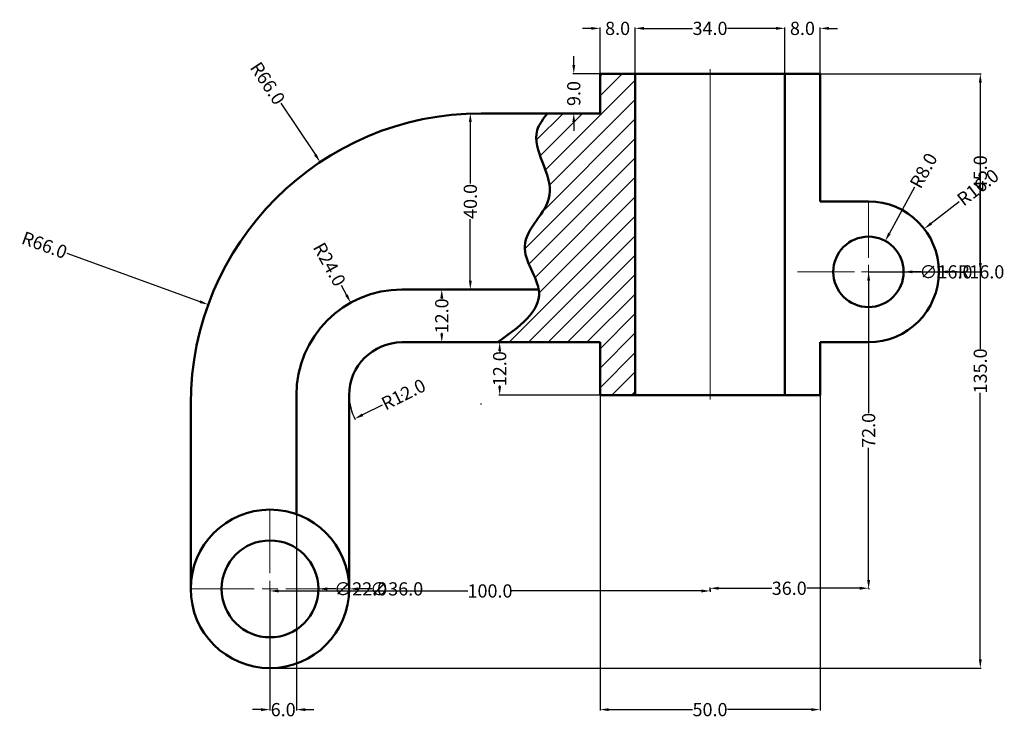
# Model space of a CAD drawing. Units: inches. Extents: x 196 to 456, y 125 to 440.
# Tile 1 of 2: x 196 to 420, y 125 to 284. Entities that reach past the tile are written whole.
import ezdxf

# ---------------------------------------------------------------- set-up
doc = ezdxf.new("R2010")
doc.units = ezdxf.units.IN
doc.header["$MEASUREMENT"] = 0
doc.linetypes.add('CENTER', pattern=[50.8, 31.75, -6.35, 6.35, -6.35])
for name, color, linetype, lineweight in [('M-CNTR', 1, 'CENTER', 18), ('M-DIMS', 2, 'Continuous', 25), ('M-HATC', 8, 'Continuous', 18), ('M-OUTL', 7, 'Continuous', 50)]:
    doc.layers.add(name, color=color, linetype=linetype, lineweight=lineweight)
doc.styles.get("Standard").update_dxf_attribs({"font": 'arial.ttf'})
doc.dimstyles.get("Standard").update_dxf_attribs({"dimtxt": 3, "dimasz": 2, "dimexe": 0.18, "dimexo": 0.0625, "dimgap": 0.09, "dimtad": 0, "dimdec": 1, "dimzin": 0, "dimdsep": 46, "dimtxsty": 'Standard', "dimcen": 0.09, "dimadec": 0, "dimazin": 0, "dimtfac": 1, "dimtdec": 1, "dimtofl": 0, "dimtmove": 0, "dimatfit": 3, "dimfxl": 1, "dimtolj": 1, "dimtzin": 0, "dimarcsym": 0})

# ---------------------------------------------------------------- blocks, each defined once
blk = doc.blocks.new('*U2')
at = {"layer": 'M-CNTR', "color": 0, "transparency": 16777216}
for p, q in [((0, 3.2), (0, 16.12)), ((-16.12, 0), (-3.2, 0)), ((3.2, 0), (16.12, 0)), ((0, -16.12), (0, -3.2))]:
    blk.add_line(p, q, dxfattribs=at)
at = {"layer": 'M-CNTR', "color": 0, "linetype": 'Continuous', "transparency": 16777216}
for p, q in [((-1.6, 0), (1.6, 0)), ((0, -1.6), (0, 1.6))]:
    blk.add_line(p, q, dxfattribs=at)
blk = doc.blocks.new('*U3')
at = {"layer": 'M-CNTR', "color": 0, "transparency": 16777216}
for p, q in [((0, 3.6), (0, 18.12)), ((-18.12, 0), (-3.6, 0)), ((3.6, 0), (18.12, 0)), ((0, -18.12), (0, -3.6))]:
    blk.add_line(p, q, dxfattribs=at)
at = {"layer": 'M-CNTR', "color": 0, "linetype": 'Continuous', "transparency": 16777216}
for p, q in [((-1.8, 0), (1.8, 0)), ((0, -1.8), (0, 1.8))]:
    blk.add_line(p, q, dxfattribs=at)
blk = doc.blocks.new('*U4')
at = {"layer": 'M-CNTR', "color": 0, "ltscale": 8, "transparency": 16777216}
blk.add_line((0, -37.5), (0, 37.5), dxfattribs=at)
blk = doc.blocks.new('*D11')
at = {"layer": 'Defpoints', "color": 0, "transparency": 16777216}
for p in [(389.31, 226.45), (389.31, 154.45), (389.35, 154.45)]:
    blk.add_point(p, dxfattribs=at)
at = {"layer": 'M-DIMS', "color": 0, "lineweight": -2, "transparency": 16777216}
for p, q in [((389.37, 226.45), (389.53, 226.45)), ((389.35, 224.45), (389.35, 194.42)), ((389.35, 156.45), (389.35, 186.48)), ((389.37, 154.45), (389.53, 154.45))]:
    blk.add_line(p, q, dxfattribs=at)
at = {"layer": 'M-DIMS', "color": 0, "transparency": 16777216}
for points in [[(389.02, 224.45), (389.69, 224.45), (389.35, 226.45)], [(389.02, 156.45), (389.69, 156.45), (389.35, 154.45)]]:
    blk.add_solid(points, dxfattribs=at)
at = {"layer": 'M-DIMS', "color": 0, "transparency": 16777216, "insert": (389.35, 190.45), "char_height": 3, "attachment_point": 5, "rotation": 90}
blk.add_mtext('\\A1;72.0', dxfattribs=at)
blk = doc.blocks.new('*D12')
at = {"layer": 'Defpoints', "color": 0, "transparency": 16777216}
for p in [(253.31, 154.45), (353.31, 154.45), (353.31, 153.98)]:
    blk.add_point(p, dxfattribs=at)
at = {"layer": 'M-DIMS', "color": 0, "lineweight": -2, "transparency": 16777216}
for p, q in [((253.31, 154.39), (253.31, 153.8)), ((353.31, 154.39), (353.31, 153.8)), ((255.31, 153.98), (298.3, 153.98)), ((351.31, 153.98), (308.31, 153.98))]:
    blk.add_line(p, q, dxfattribs=at)
at = {"layer": 'M-DIMS', "color": 0, "transparency": 16777216}
for points in [[(255.31, 154.31), (255.31, 153.64), (253.31, 153.98)], [(351.31, 154.31), (351.31, 153.64), (353.31, 153.98)]]:
    blk.add_solid(points, dxfattribs=at)
at = {"layer": 'M-DIMS', "color": 0, "transparency": 16777216, "insert": (303.31, 153.98), "char_height": 3, "attachment_point": 5}
blk.add_mtext('\\A1;100.0', dxfattribs=at)
blk = doc.blocks.new('*D13')
at = {"layer": 'Defpoints', "color": 0, "transparency": 16777216}
for p in [(389.31, 154.59), (389.31, 154.45), (353.31, 153.98)]:
    blk.add_point(p, dxfattribs=at)
at = {"layer": 'M-DIMS', "color": 0, "lineweight": -2, "transparency": 16777216}
for p, q in [((353.31, 154.04), (353.31, 154.77)), ((355.31, 154.59), (367.33, 154.59)), ((387.31, 154.59), (375.29, 154.59)), ((389.31, 154.51), (389.31, 154.77))]:
    blk.add_line(p, q, dxfattribs=at)
at = {"layer": 'M-DIMS', "color": 0, "transparency": 16777216}
for points in [[(355.31, 154.93), (355.31, 154.26), (353.31, 154.59)], [(387.31, 154.93), (387.31, 154.26), (389.31, 154.59)]]:
    blk.add_solid(points, dxfattribs=at)
at = {"layer": 'M-DIMS', "color": 0, "transparency": 16777216, "insert": (371.31, 154.59), "char_height": 3, "attachment_point": 5}
blk.add_mtext('\\A1;36.0', dxfattribs=at)
blk = doc.blocks.new('*D14')
at = {"layer": 'Defpoints', "color": 0, "transparency": 16777216}
for p in [(264.73, 251.38), (301.31, 196.45)]:
    blk.add_point(p, dxfattribs=at)
at = {"layer": 'M-DIMS', "color": 0, "lineweight": -2, "transparency": 16777216}
for p, q in [((255.81, 264.78), (263.62, 253.05)), ((301.22, 196.45), (301.4, 196.45)), ((301.31, 196.36), (301.31, 196.54))]:
    blk.add_line(p, q, dxfattribs=at)
at = {"layer": 'M-DIMS', "color": 0, "transparency": 16777216}
blk.add_solid([(263.89, 253.23), (263.34, 252.86), (264.73, 251.38)], dxfattribs=at)
at = {"layer": 'M-DIMS', "color": 0, "transparency": 16777216, "insert": (252.8, 269.28), "char_height": 3, "attachment_point": 5, "rotation": 303.6615}
blk.add_mtext('\\A1;R66.0', dxfattribs=at)
blk = doc.blocks.new('*D15')
at = {"layer": 'Defpoints', "color": 0, "transparency": 16777216}
for p in [(271.67, 219.44), (283.31, 198.45)]:
    blk.add_point(p, dxfattribs=at)
at = {"layer": 'M-DIMS', "color": 0, "lineweight": -2, "transparency": 16777216}
for p, q in [((269.47, 223.42), (270.7, 221.19)), ((283.22, 198.45), (283.4, 198.45)), ((283.31, 198.36), (283.31, 198.54))]:
    blk.add_line(p, q, dxfattribs=at)
at = {"layer": 'M-DIMS', "color": 0, "transparency": 16777216}
blk.add_solid([(270.99, 221.35), (270.41, 221.03), (271.67, 219.44)], dxfattribs=at)
at = {"layer": 'M-DIMS', "color": 0, "transparency": 16777216, "insert": (266.84, 228.15), "char_height": 3, "attachment_point": 5, "rotation": 299.0067}
blk.add_mtext('\\A1;R24.0', dxfattribs=at)
blk = doc.blocks.new('*D16')
at = {"layer": 'Defpoints', "color": 0, "transparency": 16777216}
for p in [(283.31, 198.45), (272.57, 193.09)]:
    blk.add_point(p, dxfattribs=at)
at = {"layer": 'M-DIMS', "color": 0, "lineweight": -2, "transparency": 16777216}
blk.add_line((278.81, 196.2), (274.36, 193.98), dxfattribs=at)
blk.add_arc((283.31, 198.45), 12, 180.2984, 207.4059, dxfattribs=at)
at = {"layer": 'M-DIMS', "color": 0, "transparency": 16777216}
blk.add_solid([(274.21, 194.28), (274.51, 193.68), (272.57, 193.09)], dxfattribs=at)
at = {"layer": 'M-DIMS', "color": 0, "transparency": 16777216, "insert": (283.65, 198.62), "char_height": 3, "attachment_point": 5, "rotation": 26.5465}
blk.add_mtext('\\A1;R12.0', dxfattribs=at)
blk = doc.blocks.new('*D17')
at = {"layer": 'Defpoints', "color": 0, "transparency": 16777216}
for p in [(401.98, 236.22), (389.31, 226.45)]:
    blk.add_point(p, dxfattribs=at)
at = {"layer": 'M-DIMS', "color": 0, "lineweight": -2, "transparency": 16777216}
for p, q in [((409.9, 242.34), (403.56, 237.45)), ((389.22, 226.45), (389.4, 226.45)), ((389.31, 226.36), (389.31, 226.54))]:
    blk.add_line(p, q, dxfattribs=at)
at = {"layer": 'M-DIMS', "color": 0, "transparency": 16777216}
blk.add_solid([(403.36, 237.71), (403.76, 237.18), (401.98, 236.22)], dxfattribs=at)
at = {"layer": 'M-DIMS', "color": 0, "transparency": 16777216, "insert": (414.19, 245.65), "char_height": 3, "attachment_point": 5, "rotation": 37.6579}
blk.add_mtext('\\A1;R16.0', dxfattribs=at)
blk = doc.blocks.new('*D18')
at = {"layer": 'Defpoints', "color": 0, "transparency": 16777216}
for p in [(393.14, 233.47), (389.31, 226.45)]:
    blk.add_point(p, dxfattribs=at)
at = {"layer": 'M-DIMS', "color": 0, "lineweight": -2, "transparency": 16777216}
for p, q in [((399.81, 245.72), (394.09, 235.23)), ((389.22, 226.45), (389.4, 226.45)), ((389.31, 226.36), (389.31, 226.54))]:
    blk.add_line(p, q, dxfattribs=at)
at = {"layer": 'M-DIMS', "color": 0, "transparency": 16777216}
blk.add_solid([(393.8, 235.39), (394.39, 235.07), (393.14, 233.47)], dxfattribs=at)
at = {"layer": 'M-DIMS', "color": 0, "transparency": 16777216, "insert": (401.84, 249.45), "char_height": 3, "attachment_point": 5, "rotation": 61.4164}
blk.add_mtext('\\A1;R8.0', dxfattribs=at)
blk = doc.blocks.new('*D19')
at = {"layer": 'Defpoints', "color": 0, "transparency": 16777216}
for p in [(301.31, 262.45), (298.84, 222.45), (301.31, 222.45)]:
    blk.add_point(p, dxfattribs=at)
at = {"layer": 'M-DIMS', "color": 0, "lineweight": -2, "transparency": 16777216}
for p, q in [((301.25, 262.45), (298.66, 262.45)), ((298.84, 260.45), (298.84, 246.49)), ((298.84, 224.45), (298.84, 238.41)), ((301.25, 222.45), (298.66, 222.45))]:
    blk.add_line(p, q, dxfattribs=at)
at = {"layer": 'M-DIMS', "color": 0, "transparency": 16777216}
for points in [[(298.51, 260.45), (299.18, 260.45), (298.84, 262.45)], [(298.51, 224.45), (299.18, 224.45), (298.84, 222.45)]]:
    blk.add_solid(points, dxfattribs=at)
at = {"layer": 'M-DIMS', "color": 0, "transparency": 16777216, "insert": (298.84, 242.45), "char_height": 3, "attachment_point": 5, "rotation": 90}
blk.add_mtext('\\A1;40.0', dxfattribs=at)
blk = doc.blocks.new('*D20')
at = {"layer": 'Defpoints', "color": 0, "transparency": 16777216}
for p in [(292.35, 222.45), (298.84, 222.45), (298.84, 210.45)]:
    blk.add_point(p, dxfattribs=at)
at = {"layer": 'M-DIMS', "color": 0, "lineweight": -2, "transparency": 16777216}
for p, q in [((298.78, 222.45), (292.17, 222.45)), ((292.35, 220.45), (292.35, 220.29)), ((292.35, 212.45), (292.35, 212.61)), ((298.78, 210.45), (292.17, 210.45))]:
    blk.add_line(p, q, dxfattribs=at)
at = {"layer": 'M-DIMS', "color": 0, "transparency": 16777216}
for points in [[(292.02, 220.45), (292.69, 220.45), (292.35, 222.45)], [(292.02, 212.45), (292.69, 212.45), (292.35, 210.45)]]:
    blk.add_solid(points, dxfattribs=at)
at = {"layer": 'M-DIMS', "color": 0, "transparency": 16777216, "insert": (292.35, 216.45), "char_height": 3, "attachment_point": 5, "rotation": 90}
blk.add_mtext('\\A1;12.0', dxfattribs=at)
blk = doc.blocks.new('*D21')
at = {"layer": 'Defpoints', "color": 0, "transparency": 16777216}
for p in [(328.31, 210.45), (305.51, 198.45), (328.31, 198.45)]:
    blk.add_point(p, dxfattribs=at)
at = {"layer": 'M-DIMS', "color": 0, "lineweight": -2, "transparency": 16777216}
for p, q in [((328.25, 210.45), (305.33, 210.45)), ((305.51, 208.45), (305.51, 208.29)), ((305.51, 200.45), (305.51, 200.61)), ((328.25, 198.45), (305.33, 198.45))]:
    blk.add_line(p, q, dxfattribs=at)
at = {"layer": 'M-DIMS', "color": 0, "transparency": 16777216}
for points in [[(305.18, 208.45), (305.84, 208.45), (305.51, 210.45)], [(305.18, 200.45), (305.84, 200.45), (305.51, 198.45)]]:
    blk.add_solid(points, dxfattribs=at)
at = {"layer": 'M-DIMS', "color": 0, "transparency": 16777216, "insert": (305.51, 204.45), "char_height": 3, "attachment_point": 5, "rotation": 90}
blk.add_mtext('\\A1;12.0', dxfattribs=at)
blk = doc.blocks.new('*D22')
at = {"layer": 'Defpoints', "color": 0, "transparency": 16777216}
for p in [(328.31, 271.45), (322.35, 262.45), (328.31, 262.45)]:
    blk.add_point(p, dxfattribs=at)
at = {"layer": 'M-DIMS', "color": 0, "lineweight": -2, "transparency": 16777216}
for p, q in [((322.35, 273.45), (322.35, 275.45)), ((328.25, 271.45), (322.17, 271.45)), ((328.25, 262.45), (322.17, 262.45)), ((322.35, 260.45), (322.35, 258.45))]:
    blk.add_line(p, q, dxfattribs=at)
at = {"layer": 'M-DIMS', "color": 0, "transparency": 16777216}
for points in [[(322.02, 273.45), (322.68, 273.45), (322.35, 271.45)], [(322.02, 260.45), (322.68, 260.45), (322.35, 262.45)]]:
    blk.add_solid(points, dxfattribs=at)
at = {"layer": 'M-DIMS', "color": 0, "transparency": 16777216, "insert": (322.35, 266.95), "char_height": 3, "attachment_point": 5, "rotation": 90}
blk.add_mtext('\\A1;9.0', dxfattribs=at)
blk = doc.blocks.new('*D24')
at = {"layer": 'Defpoints', "color": 0, "transparency": 16777216}
for p in [(328.31, 198.45), (378.31, 198.45), (378.31, 127.03)]:
    blk.add_point(p, dxfattribs=at)
at = {"layer": 'M-DIMS', "color": 0, "lineweight": -2, "transparency": 16777216}
for p, q in [((328.31, 198.39), (328.31, 126.85)), ((378.31, 198.39), (378.31, 126.85)), ((330.31, 127.03), (349.33, 127.03)), ((376.31, 127.03), (357.29, 127.03))]:
    blk.add_line(p, q, dxfattribs=at)
at = {"layer": 'M-DIMS', "color": 0, "transparency": 16777216}
for points in [[(330.31, 127.36), (330.31, 126.7), (328.31, 127.03)], [(376.31, 127.36), (376.31, 126.7), (378.31, 127.03)]]:
    blk.add_solid(points, dxfattribs=at)
at = {"layer": 'M-DIMS', "color": 0, "transparency": 16777216, "insert": (353.31, 127.03), "char_height": 3, "attachment_point": 5}
blk.add_mtext('\\A1;50.0', dxfattribs=at)
blk = doc.blocks.new('*D25')
at = {"layer": 'Defpoints', "color": 0, "transparency": 16777216}
for p in [(336.31, 281.75), (328.31, 271.45), (336.31, 271.45)]:
    blk.add_point(p, dxfattribs=at)
at = {"layer": 'M-DIMS', "color": 0, "lineweight": -2, "transparency": 16777216}
for p, q in [((328.31, 271.51), (328.31, 281.93)), ((336.31, 271.51), (336.31, 281.93)), ((326.31, 281.75), (324.31, 281.75)), ((338.31, 281.75), (340.31, 281.75))]:
    blk.add_line(p, q, dxfattribs=at)
at = {"layer": 'M-DIMS', "color": 0, "transparency": 16777216}
for points in [[(326.31, 282.08), (326.31, 281.42), (328.31, 281.75)], [(338.31, 282.08), (338.31, 281.42), (336.31, 281.75)]]:
    blk.add_solid(points, dxfattribs=at)
at = {"layer": 'M-DIMS', "color": 0, "transparency": 16777216, "insert": (332.31, 281.75), "char_height": 3, "attachment_point": 5}
blk.add_mtext('\\A1;8.0', dxfattribs=at)
blk = doc.blocks.new('*D26')
at = {"layer": 'Defpoints', "color": 0, "transparency": 16777216}
for p in [(370.31, 281.75), (336.31, 271.45), (370.31, 271.45)]:
    blk.add_point(p, dxfattribs=at)
at = {"layer": 'M-DIMS', "color": 0, "lineweight": -2, "transparency": 16777216}
for p, q in [((336.31, 271.51), (336.31, 281.93)), ((370.31, 271.51), (370.31, 281.93)), ((338.31, 281.75), (349.33, 281.75)), ((368.31, 281.75), (357.29, 281.75))]:
    blk.add_line(p, q, dxfattribs=at)
at = {"layer": 'M-DIMS', "color": 0, "transparency": 16777216}
for points in [[(338.31, 282.08), (338.31, 281.42), (336.31, 281.75)], [(368.31, 282.08), (368.31, 281.42), (370.31, 281.75)]]:
    blk.add_solid(points, dxfattribs=at)
at = {"layer": 'M-DIMS', "color": 0, "transparency": 16777216, "insert": (353.31, 281.75), "char_height": 3, "attachment_point": 5}
blk.add_mtext('\\A1;34.0', dxfattribs=at)
blk = doc.blocks.new('*D27')
at = {"layer": 'Defpoints', "color": 0, "transparency": 16777216}
for p in [(378.31, 281.75), (370.31, 271.45), (378.31, 271.45)]:
    blk.add_point(p, dxfattribs=at)
at = {"layer": 'M-DIMS', "color": 0, "lineweight": -2, "transparency": 16777216}
for p, q in [((370.31, 271.51), (370.31, 281.93)), ((378.31, 271.51), (378.31, 281.93)), ((368.31, 281.75), (366.31, 281.75)), ((380.31, 281.75), (382.31, 281.75))]:
    blk.add_line(p, q, dxfattribs=at)
at = {"layer": 'M-DIMS', "color": 0, "transparency": 16777216}
for points in [[(368.31, 282.08), (368.31, 281.42), (370.31, 281.75)], [(380.31, 282.08), (380.31, 281.42), (378.31, 281.75)]]:
    blk.add_solid(points, dxfattribs=at)
at = {"layer": 'M-DIMS', "color": 0, "transparency": 16777216, "insert": (374.31, 281.75), "char_height": 3, "attachment_point": 5}
blk.add_mtext('\\A1;8.0', dxfattribs=at)
blk = doc.blocks.new('*D28')
at = {"layer": 'Defpoints', "color": 0, "transparency": 16777216}
for p in [(378.31, 271.45), (414.73, 271.45), (389.31, 226.45)]:
    blk.add_point(p, dxfattribs=at)
at = {"layer": 'M-DIMS', "color": 0, "lineweight": -2, "transparency": 16777216}
for p, q in [((378.37, 271.45), (414.91, 271.45)), ((414.73, 269.45), (414.73, 252.99)), ((414.73, 228.45), (414.73, 244.91)), ((389.37, 226.45), (414.91, 226.45))]:
    blk.add_line(p, q, dxfattribs=at)
at = {"layer": 'M-DIMS', "color": 0, "transparency": 16777216}
for points in [[(414.4, 269.45), (415.06, 269.45), (414.73, 271.45)], [(414.4, 228.45), (415.06, 228.45), (414.73, 226.45)]]:
    blk.add_solid(points, dxfattribs=at)
at = {"layer": 'M-DIMS', "color": 0, "transparency": 16777216, "insert": (414.73, 248.95), "char_height": 3, "attachment_point": 5, "rotation": 90}
blk.add_mtext('\\A1;45.0', dxfattribs=at)
blk = doc.blocks.new('*D29')
at = {"layer": 'Defpoints', "color": 0, "transparency": 16777216}
for p in [(259.31, 171.42), (253.31, 154.45), (259.31, 127.03)]:
    blk.add_point(p, dxfattribs=at)
at = {"layer": 'M-DIMS', "color": 0, "lineweight": -2, "transparency": 16777216}
for p, q in [((259.31, 171.36), (259.31, 126.85)), ((253.31, 154.39), (253.31, 126.85)), ((251.31, 127.03), (249.31, 127.03)), ((261.31, 127.03), (263.31, 127.03))]:
    blk.add_line(p, q, dxfattribs=at)
at = {"layer": 'M-DIMS', "color": 0, "transparency": 16777216}
for points in [[(251.31, 127.36), (251.31, 126.7), (253.31, 127.03)], [(261.31, 127.36), (261.31, 126.7), (259.31, 127.03)]]:
    blk.add_solid(points, dxfattribs=at)
at = {"layer": 'M-DIMS', "color": 0, "transparency": 16777216, "insert": (256.31, 127.03), "char_height": 3, "attachment_point": 5}
blk.add_mtext('\\A1;6.0', dxfattribs=at)
blk = doc.blocks.new('*D30')
at = {"layer": 'Defpoints', "color": 0, "transparency": 16777216}
for p in [(378.31, 271.45), (414.73, 271.45), (253.31, 136.45)]:
    blk.add_point(p, dxfattribs=at)
at = {"layer": 'M-DIMS', "color": 0, "lineweight": -2, "transparency": 16777216}
for p, q in [((378.37, 271.45), (414.91, 271.45)), ((414.73, 269.45), (414.73, 208.95)), ((414.73, 138.45), (414.73, 198.94)), ((253.37, 136.45), (414.91, 136.45))]:
    blk.add_line(p, q, dxfattribs=at)
at = {"layer": 'M-DIMS', "color": 0, "transparency": 16777216}
for points in [[(414.4, 269.45), (415.06, 269.45), (414.73, 271.45)], [(414.4, 138.45), (415.06, 138.45), (414.73, 136.45)]]:
    blk.add_solid(points, dxfattribs=at)
at = {"layer": 'M-DIMS', "color": 0, "transparency": 16777216, "insert": (414.73, 203.95), "char_height": 3, "attachment_point": 5, "rotation": 90}
blk.add_mtext('\\A1;135.0', dxfattribs=at)
blk = doc.blocks.new('*D37')
at = {"layer": 'Defpoints', "color": 0, "transparency": 16777216}
for p in [(239.28, 219.01), (301.31, 196.45)]:
    blk.add_point(p, dxfattribs=at)
at = {"layer": 'M-DIMS', "color": 0, "lineweight": -2, "transparency": 16777216}
for p, q in [((207.16, 230.69), (237.4, 219.69)), ((301.22, 196.45), (301.4, 196.45)), ((301.31, 196.36), (301.31, 196.54))]:
    blk.add_line(p, q, dxfattribs=at)
at = {"layer": 'M-DIMS', "color": 0, "transparency": 16777216}
blk.add_solid([(237.52, 220), (237.29, 219.38), (239.28, 219.01)], dxfattribs=at)
at = {"layer": 'M-DIMS', "color": 0, "transparency": 16777216, "insert": (202.07, 232.54), "char_height": 3, "attachment_point": 5, "rotation": 340.015}
blk.add_mtext('\\A1;R66.0', dxfattribs=at)
blk = doc.blocks.new('*D38')
at = {"layer": 'Defpoints', "color": 0, "transparency": 16777216}
for p in [(389.31, 226.45), (405.31, 226.45)]:
    blk.add_point(p, dxfattribs=at)
at = {"layer": 'M-DIMS', "color": 0, "lineweight": -2, "transparency": 16777216}
for p, q in [((389.22, 226.45), (389.4, 226.45)), ((389.31, 226.36), (389.31, 226.54)), ((409.49, 226.45), (407.31, 226.45))]:
    blk.add_line(p, q, dxfattribs=at)
at = {"layer": 'M-DIMS', "color": 0, "transparency": 16777216}
blk.add_solid([(407.31, 226.78), (407.31, 226.12), (405.31, 226.45)], dxfattribs=at)
at = {"layer": 'M-DIMS', "color": 0, "transparency": 16777216, "insert": (414.91, 226.45), "char_height": 3, "attachment_point": 5, "rotation": 359.9996}
blk.add_mtext('\\A1;R16.0', dxfattribs=at)
blk = doc.blocks.new('*D39')
at = {"layer": 'Defpoints', "color": 0, "transparency": 16777216}
for p in [(381.31, 226.45), (397.31, 226.45)]:
    blk.add_point(p, dxfattribs=at)
at = {"layer": 'M-DIMS', "color": 0, "lineweight": -2, "transparency": 16777216}
for p, q in [((389.22, 226.45), (389.4, 226.45)), ((389.31, 226.36), (389.31, 226.54)), ((401.31, 226.45), (399.31, 226.45))]:
    blk.add_line(p, q, dxfattribs=at)
at = {"layer": 'M-DIMS', "color": 0, "transparency": 16777216}
blk.add_solid([(399.31, 226.78), (399.31, 226.12), (397.31, 226.45)], dxfattribs=at)
at = {"layer": 'M-DIMS', "color": 0, "transparency": 16777216, "insert": (406.92, 226.45), "char_height": 3, "attachment_point": 5, "rotation": 359.9992}
blk.add_mtext('\\A1;∅16.0', dxfattribs=at)
blk = doc.blocks.new('*D40')
at = {"layer": 'Defpoints', "color": 0, "transparency": 16777216}
for p in [(235.31, 154.45), (271.31, 154.45)]:
    blk.add_point(p, dxfattribs=at)
at = {"layer": 'M-DIMS', "color": 0, "lineweight": -2, "transparency": 16777216}
for p, q in [((253.22, 154.45), (253.4, 154.45)), ((253.31, 154.36), (253.31, 154.54)), ((276.5, 154.45), (273.31, 154.45))]:
    blk.add_line(p, q, dxfattribs=at)
at = {"layer": 'M-DIMS', "color": 0, "transparency": 16777216}
blk.add_solid([(273.31, 154.78), (273.31, 154.12), (271.31, 154.45)], dxfattribs=at)
at = {"layer": 'M-DIMS', "color": 0, "transparency": 16777216, "insert": (282.11, 154.45), "char_height": 3, "attachment_point": 5, "rotation": 359.9996}
blk.add_mtext('\\A1;∅36.0', dxfattribs=at)
blk = doc.blocks.new('*D41')
at = {"layer": 'Defpoints', "color": 0, "transparency": 16777216}
for p in [(242.31, 154.45), (264.31, 154.45)]:
    blk.add_point(p, dxfattribs=at)
at = {"layer": 'M-DIMS', "color": 0, "lineweight": -2, "transparency": 16777216}
for p, q in [((253.22, 154.45), (253.4, 154.45)), ((253.31, 154.36), (253.31, 154.54)), ((268.31, 154.45), (266.31, 154.45))]:
    blk.add_line(p, q, dxfattribs=at)
at = {"layer": 'M-DIMS', "color": 0, "transparency": 16777216}
blk.add_solid([(266.31, 154.78), (266.31, 154.12), (264.31, 154.45)], dxfattribs=at)
at = {"layer": 'M-DIMS', "color": 0, "transparency": 16777216, "insert": (273.92, 154.45), "char_height": 3, "attachment_point": 5, "rotation": 359.9994}
blk.add_mtext('\\A1;∅22.0', dxfattribs=at)

msp = doc.modelspace()

# ---------------------------------------------------------------- hatches: boundary and pattern name
at = {"layer": 'M-HATC'}
h = msp.add_hatch(dxfattribs=at)
h.set_pattern_fill('ANSI31', color=256, scale=25)
edge = h.paths.add_edge_path()
edge.add_line((336.309, 271.449), (328.309, 271.449))
edge.add_line((328.309, 271.449), (328.309, 262.449))
edge.add_line((328.309, 262.449), (316.35, 262.449))
edge.add_spline(control_points=[(316.35, 262.449), (315.389, 261.196), (311.231, 255.775), (321.83, 243.899), (307.533, 233.54), (313.825, 225.58), (314.379, 222.449)], knot_values=[0, 0, 0, 0, 4.4967115, 19.4510347, 32.3564823, 42.6673107, 42.6673107, 42.6673107, 42.6673107], degree=3, periodic=0)
edge.add_spline(control_points=[(314.379, 222.449), (314.412, 222.258), (315.039, 217.6), (309.917, 213.951), (305.004, 210.449)], knot_values=[42.6673107, 42.6673107, 42.6673107, 42.6673107, 43.2952236, 58.1279215, 58.1279215, 58.1279215, 58.1279215], degree=3, periodic=0)
edge.add_line((305.004, 210.449), (328.309, 210.449))
edge.add_line((328.309, 210.449), (328.309, 198.449))
edge.add_line((328.309, 198.449), (336.309, 198.449))
edge.add_line((336.309, 198.449), (336.309, 271.449))

# ---------------------------------------------------------------- linework, layer by layer
at = {"layer": 'M-OUTL'}
for p, q in [((378.309, 271.449), (328.309, 271.449)), ((328.309, 262.449), (328.309, 271.449)), ((336.309, 198.449), (336.309, 271.449)), ((370.309, 198.449), (370.309, 271.449)), ((378.309, 242.449), (378.309, 271.449)), ((328.309, 262.449), (301.309, 262.449)), ((389.309, 242.449), (378.309, 242.449)), ((314.379, 222.449), (283.309, 222.449)), ((328.309, 210.449), (283.309, 210.449)), ((328.309, 198.449), (328.309, 210.449)), ((389.309, 210.449), (378.309, 210.449)), ((378.309, 198.449), (378.309, 210.449)), ((378.309, 198.449), (378.309, 210.449)), ((259.309, 171.42), (259.309, 198.449)), ((271.309, 154.449), (271.309, 198.449)), ((378.309, 198.449), (328.309, 198.449)), ((235.309, 154.449), (235.309, 196.449))]:
    msp.add_line(p, q, dxfattribs=at)
for centre, radius in [((389.309, 226.449), 8), ((253.309, 154.449), 18), ((253.309, 154.449), 11)]:
    msp.add_circle(centre, radius, dxfattribs=at)
for centre, radius, start, end in [((301.309, 196.449), 66, 90, 180), ((389.309, 226.449), 16, 270, 90), ((283.309, 198.449), 24, 90, 180), ((283.309, 198.449), 12, 90, 180)]:
    msp.add_arc(centre, radius, start, end, dxfattribs=at)
msp.add_open_spline([(316.35, 262.449), (315.389, 261.196), (311.231, 255.775), (321.83, 243.899), (307.298, 233.369), (318.454, 220.034), (309.917, 213.951), (305.004, 210.449)], degree=3, knots=[0, 0, 0, 0, 4.4967115, 19.4510347, 32.3564823, 43.2952236, 58.1279215, 58.1279215, 58.1279215, 58.1279215], dxfattribs=at)

# ---------------------------------------------------------------- block references
at = {"layer": 'M-CNTR', "ltscale": 8}
msp.add_blockref('*U4', (353.309, 234.949), dxfattribs=at)
at = {"layer": 'M-CNTR'}
for name, p in [('*U2', (389.309, 226.449)), ('*U3', (253.309, 154.449))]:
    msp.add_blockref(name, p, dxfattribs=at)

# ---------------------------------------------------------------- dimensions: what is measured, and where the dimension line sits
at = {"layer": 'M-DIMS'}
for base, p1, p2, override, picture, middle in [((336.309, 281.749), (328.309, 271.449), (336.309, 271.449), {"dimdec": 1, "dimlfac": 1, "dimrnd": 0, "dimzin": 0, "dimdsep": 46, "dimlunit": 2}, '*D25', (332.309, 281.749)), ((370.309, 281.749), (336.309, 271.449), (370.309, 271.449), {"dimdec": 1, "dimlfac": 1, "dimrnd": 0, "dimzin": 0, "dimdsep": 46, "dimlunit": 2}, '*D26', (353.309, 281.749)), ((378.309, 281.749), (370.309, 271.449), (378.309, 271.449), {"dimdec": 1, "dimlfac": 1, "dimrnd": 0, "dimzin": 0, "dimdsep": 46, "dimlunit": 2}, '*D27', (374.309, 281.749)), ((378.309, 127.029), (328.309, 198.449), (378.309, 198.449), {"dimdec": 1, "dimlfac": 1, "dimrnd": 0, "dimzin": 0, "dimdsep": 46, "dimlunit": 2}, '*D24', (353.309, 127.029)), ((259.309, 127.029), (253.309, 154.449), (259.309, 171.42), {"dimdec": 1, "dimlfac": 1, "dimrnd": 0, "dimzin": 0, "dimdsep": 46, "dimlunit": 2}, '*D29', (256.309, 127.029)), ((353.309, 153.976), (253.309, 154.449), (353.309, 154.449), {"dimclrd": 0, "dimclre": 0, "dimclrt": 0}, '*D12', (303.309, 153.976)), ((389.309, 154.595), (353.309, 153.976), (389.309, 154.449), {"dimclrd": 0, "dimclre": 0, "dimclrt": 0}, '*D13', (371.309, 154.595))]:
    dim = msp.add_linear_dim(base=base, p1=p1, p2=p2, dimstyle='Standard', override=override, dxfattribs=at)
    dim.commit()
    dim.dimension.update_dxf_attribs({"geometry": picture, "text_midpoint": middle})
for base, p1, p2, override, picture, middle in [((322.349, 262.449), (328.309, 271.449), (328.309, 262.449), {"dimclrd": 0, "dimclre": 0, "dimclrt": 0}, '*D22', (322.349, 266.949)), ((414.729, 271.449), (253.309, 136.449), (378.309, 271.449), {"dimdec": 1, "dimlfac": 1, "dimrnd": 0, "dimzin": 0, "dimdsep": 46, "dimlunit": 2}, '*D30', (414.729, 203.949)), ((414.729, 271.449), (389.309, 226.449), (378.309, 271.449), {"dimdec": 1, "dimlfac": 1, "dimrnd": 0, "dimzin": 0, "dimdsep": 46, "dimlunit": 2}, '*D28', (414.729, 248.949)), ((298.844, 222.449), (301.309, 262.449), (301.309, 222.449), {"dimclrd": 0, "dimclre": 0, "dimclrt": 0}, '*D19', (298.844, 242.449)), ((389.353, 154.449), (389.309, 226.449), (389.309, 154.449), {"dimclrd": 0, "dimclre": 0, "dimclrt": 0}, '*D11', (389.353, 190.449)), ((292.354, 222.449), (298.844, 210.449), (298.844, 222.449), {"dimclrd": 0, "dimclre": 0, "dimclrt": 0}, '*D20', (292.354, 216.449)), ((305.511, 198.449), (328.309, 210.449), (328.309, 198.449), {"dimclrd": 0, "dimclre": 0, "dimclrt": 0}, '*D21', (305.511, 204.449))]:
    dim = msp.add_linear_dim(base=base, p1=p1, p2=p2, angle=90, dimstyle='Standard', override=override, dxfattribs=at)
    dim.commit()
    dim.dimension.update_dxf_attribs({"geometry": picture, "text_midpoint": middle})
for center, mpoint, override, picture, middle in [((301.309, 196.449), (264.726, 251.383), {"dimclrd": 0, "dimclre": 0, "dimclrt": 0}, '*D14', (252.804, 269.285)), ((389.309, 226.449), (393.136, 233.474), {"dimclrd": 0, "dimclre": 0, "dimclrt": 0}, '*D18', (401.841, 249.45)), ((389.309, 226.449), (401.975, 236.224), {"dimclrd": 0, "dimclre": 0, "dimclrt": 0}, '*D17', (414.191, 245.651)), ((301.309, 196.449), (239.283, 219.006), {"dimdec": 1, "dimlfac": 1, "dimrnd": 0, "dimzin": 0, "dimdsep": 46, "dimlunit": 2}, '*D37', (202.068, 232.54)), ((283.309, 198.449), (271.671, 219.439), {"dimclrd": 0, "dimclre": 0, "dimclrt": 0}, '*D15', (266.839, 228.153)), ((389.309, 226.449), (405.309, 226.449), {"dimdec": 1, "dimlfac": 1, "dimrnd": 0, "dimzin": 0, "dimdsep": 46, "dimlunit": 2}, '*D38', (414.909, 226.449)), ((283.309, 198.449), (272.574, 193.086), {"dimclrd": 0, "dimclre": 0, "dimclrt": 0}, '*D16', (283.651, 198.62))]:
    dim = msp.add_radius_dim(center=center, mpoint=mpoint, dimstyle='Standard', override=override, dxfattribs=at)
    dim.commit()
    dim.dimension.update_dxf_attribs({"geometry": picture, "text_midpoint": middle, "dimtype": 164})
for p1, p2, picture, middle in [((381.309, 226.449), (397.309, 226.449), '*D39', (406.922, 226.449)), ((235.309, 154.449), (271.309, 154.449), '*D40', (282.109, 154.449)), ((242.309, 154.449), (264.309, 154.449), '*D41', (273.922, 154.449))]:
    dim = msp.add_diameter_dim_2p(p1=p1, p2=p2, dimstyle='Standard', override={"dimdec": 1, "dimlfac": 1, "dimrnd": 0, "dimzin": 0, "dimdsep": 46, "dimlunit": 2}, dxfattribs=at)
    dim.commit()
    dim.dimension.update_dxf_attribs({"geometry": picture, "text_midpoint": middle, "dimtype": 163})

doc.saveas('drawing.dxf')
